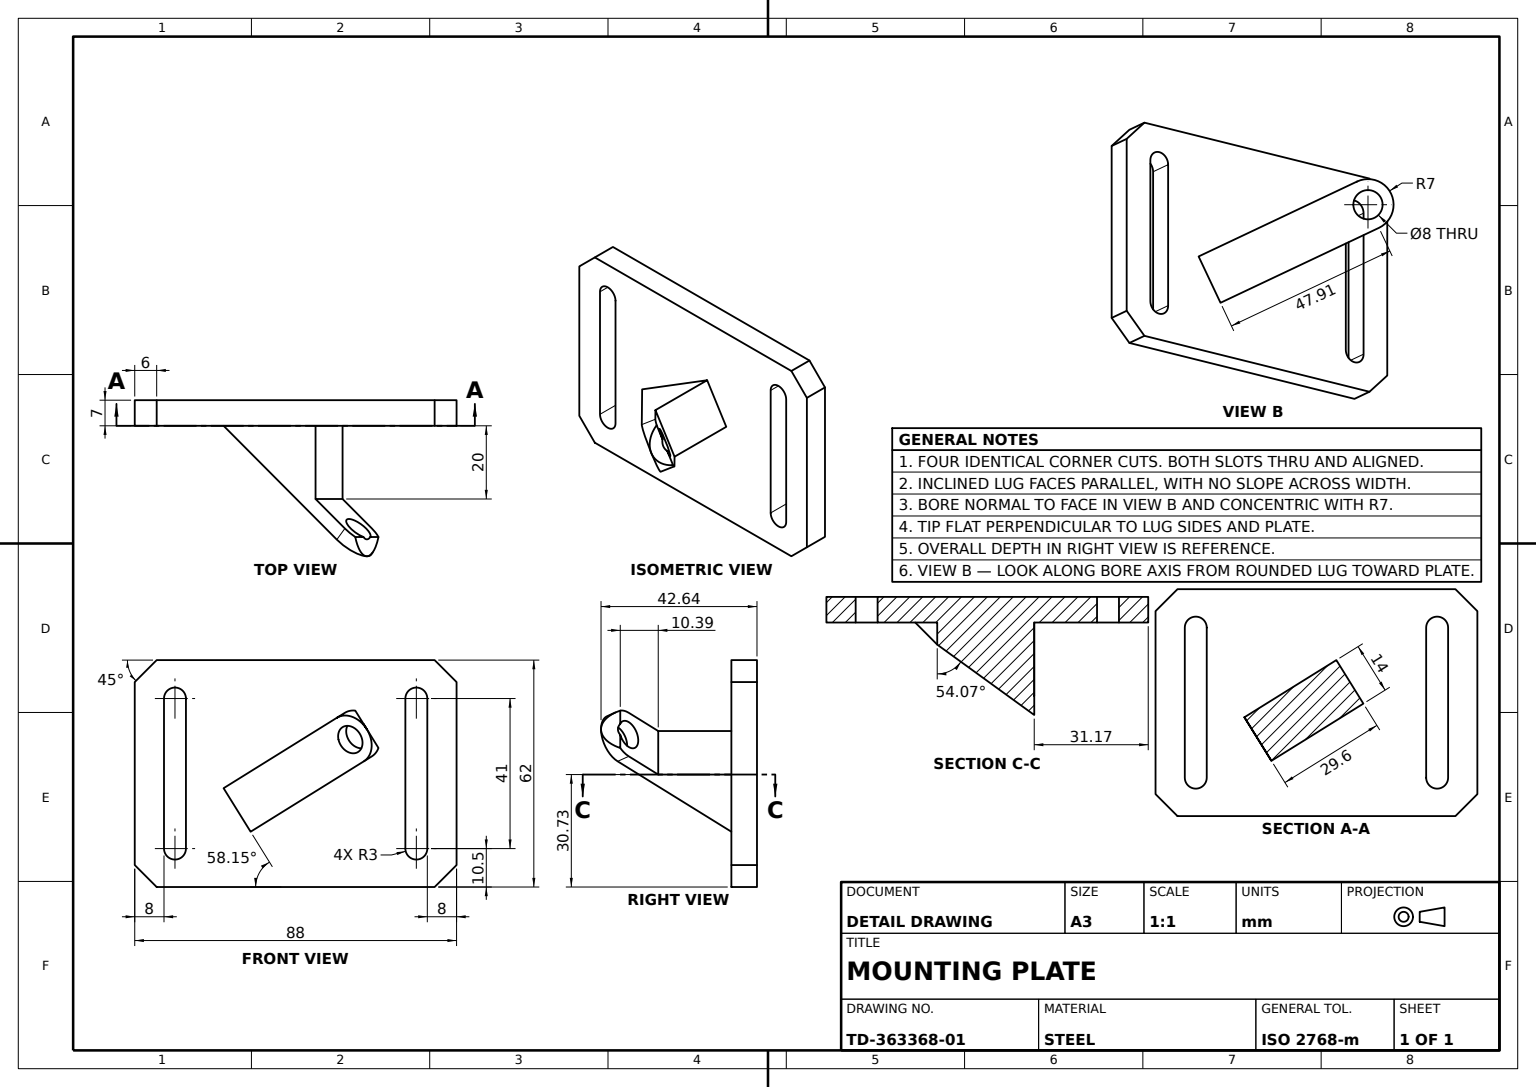
from build123d import *

# Parameters (mm, degrees)
BASE_PLATE_DEPTH            = 7
ANGLED_BLOCK_DEPTH          = 50
BLOCK_NOTCH_CUT_DEPTH       = 74.464277033
BLOCK_NOTCH_CUT_DEPTH_BACK  = 74.464277033
BLOCK_RECESS_CUT_DEPTH      = 72.480306495
BLOCK_RECESS_CUT_DEPTH_BACK = 13
BLOCK_RECESS_SKETCH_R       = 4


with BuildPart() as part:
    # Base Plate Sketch → Base Plate (new body)
    with BuildSketch(Plane.XY):
        Polygon((-44, 25), (-38, 31), (38, 31), (44, 25), (44, -25), (38, -31), (-38, -31), (-44, -25), align=None)
        with BuildLine():
            Line((-30, 20.5), (-30, -20.5))
            ThreePointArc((-30, -20.5), (-33, -23.5), (-36, -20.5))
            Line((-36, -20.5), (-36, 20.5))
            ThreePointArc((-36, 20.5), (-33, 23.5), (-30, 20.5))
        make_face(mode=Mode.SUBTRACT)
        with BuildLine():
            Line((36, 20.5), (36, -20.5))
            ThreePointArc((36, -20.5), (33, -23.5), (30, -20.5))
            Line((30, -20.5), (30, 20.5))
            ThreePointArc((30, 20.5), (33, 23.5), (36, 20.5))
        make_face(mode=Mode.SUBTRACT)
    extrude(amount=BASE_PLATE_DEPTH)

    # Angled Block Sketch → Angled Block (add)
    with BuildSketch(Plane.XY):
        Polygon((-19.704957389, -4.000247215), (-12.317392569, -15.892424729), (23.166882613, 6.150837127), (15.779317794, 18.043014641), align=None)
    extrude(amount=ANGLED_BLOCK_DEPTH)

    # Block Notch Sketch → Block Notch Cut (cut, two sides: drawn at the far end of the back side and taken through both)
    with BuildSketch(Plane(origin=(0, 0, 0), x_dir=(0.8494412510349073, 0.5276832014004726, 0), z_dir=(0.5276832014004726, -0.8494412510349073, 0)).offset(-BLOCK_NOTCH_CUT_DEPTH_BACK)):
        Polygon((-18.849066913, 50), (-18.849066913, 7), (22.924599176, 42.643551505), (22.924599176, 50), align=None)
        Polygon((10.753136621, 27), (10.753136621, 7), (15.483777963, 7), (22.924599176, 7), (22.924599176, 37.385350224), align=None)
    extrude(amount=BLOCK_NOTCH_CUT_DEPTH + BLOCK_NOTCH_CUT_DEPTH_BACK, mode=Mode.SUBTRACT)

    # Block Recess Sketch → Block Recess Cut (cut, two sides: drawn at the far end of the back side and taken through both)
    with BuildSketch(Plane(origin=(-9.681672009, -6.014372005, 13.357913864), x_dir=(0.8342680576474281, -0.22636189915410374, 0.5027495386378142), z_dir=(-0.5513590554159673, -0.3425109283644645, 0.7607164096834806)).offset(-BLOCK_RECESS_CUT_DEPTH_BACK)):
        with Locations(Location((29.524664999, 24.110272289, 0), (0, 0, 193.941739612))):
            Circle(BLOCK_RECESS_SKETCH_R)
        with BuildLine():
            ThreePointArc((36.524664999, 24.110272289), (35.848943941, 21.109689701), (33.952237609, 18.688409068))
            Line((33.952237609, 18.688409068), (39.374100831, 23.115981696))
            Line((39.374100831, 23.115981696), (34.946528251, 28.53784486))
            ThreePointArc((34.946528251, 28.53784486), (36.118337828, 26.460480496), (36.524664999, 24.110272289))
        make_face()
        with BuildLine():
            Line((30.518955591, 33.959708121), (25.097092428, 29.532135541))
            ThreePointArc((25.097092428, 29.532135541), (30.227734682, 31.07487515), (34.946528251, 28.53784486))
            Line((34.946528251, 28.53784486), (30.518955591, 33.959708121))
        make_face()
    extrude(amount=BLOCK_RECESS_CUT_DEPTH + BLOCK_RECESS_CUT_DEPTH_BACK, mode=Mode.SUBTRACT)


solid = part.part
